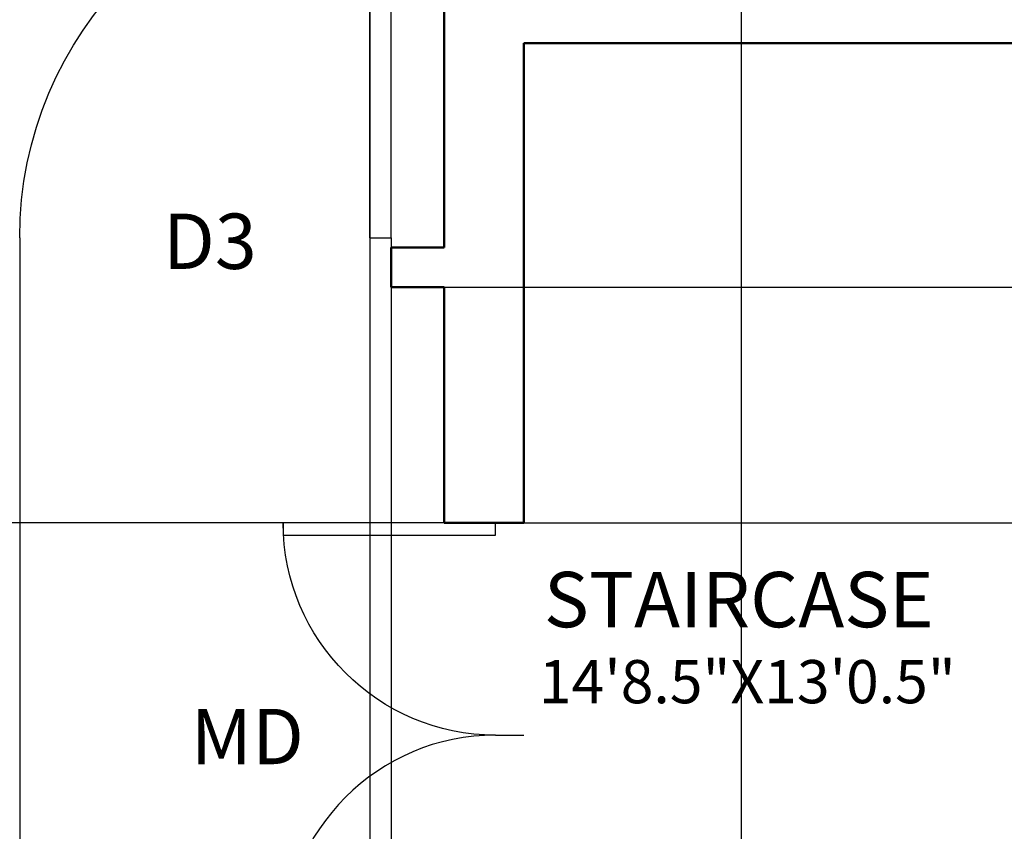
# Model space of a CAD drawing. Units: inches. Extents: x 7359 to 7979, y 33027 to 34263.
# Tile 28 of 32: x 7641 to 7753, y 33841 to 33933. Entities that reach past the tile are written whole.
import ezdxf

# ---------------------------------------------------------------- set-up
doc = ezdxf.new("R2010")
doc.units = ezdxf.units.IN
for name, color, linetype, lineweight in [('A-ANNO-DIMS', 2, 'Continuous', 18), ('A-ANNO-TEXT', 3, 'Continuous', 18), ('A-AREA-IDEN', 7, 'Continuous', 18), ('A-DOOR', 3, 'Continuous', 25), ('A-WALL', 7, 'Continuous', 50)]:
    doc.layers.add(name, color=color, linetype=linetype, lineweight=lineweight)
doc.styles.get("Standard").update_dxf_attribs({"font": 'arial.ttf'})
doc.dimstyles.get("Standard").update_dxf_attribs({"dimtxt": 0.18, "dimasz": 0.18, "dimexe": 0.18, "dimexo": 0.0625, "dimgap": 0.09, "dimtad": 0, "dimtih": 1, "dimtoh": 1, "dimdec": 4, "dimzin": 0, "dimdsep": 46, "dimtxsty": 'Standard', "dimcen": 0.09, "dimadec": 0, "dimazin": 0, "dimtfac": 1, "dimtdec": 4, "dimtofl": 0, "dimtmove": 0, "dimatfit": 3, "dimfxl": 1, "dimtolj": 1, "dimtzin": 0, "dimarcsym": 0})

# ---------------------------------------------------------------- blocks, each defined once
blk = doc.blocks.new('*U2')
for p, q in [((0, 0), (0, -100)), ((750, 0), (750, -100))]:
    blk.add_line(p, q)
blk.add_lwpolyline([(0, 0), (0, 750), (43.75, 750), (43.75, 0)], close=True)
blk.add_arc((0, 0), 750, 0, 90)
blk = doc.blocks.new('*D69')
at = {"layer": 'A-ANNO-DIMS', "color": 0, "lineweight": -2, "transparency": 16777216}
for p, q in [((7681.09, 34081.77), (7681.09, 33632.31)), ((7723.09, 34081.77), (7723.09, 33632.31)), ((7681.27, 33632.49), (7701.87, 33632.49)), ((7722.91, 33632.49), (7702.31, 33632.49))]:
    blk.add_line(p, q, dxfattribs=at)
at = {"layer": 'A-ANNO-DIMS', "color": 0, "transparency": 16777216}
for points in [[(7681.27, 33632.52), (7681.27, 33632.46), (7681.09, 33632.49)], [(7722.91, 33632.52), (7722.91, 33632.46), (7723.09, 33632.49)]]:
    blk.add_solid(points, dxfattribs=at)
at = {"layer": 'Defpoints', "color": 0, "transparency": 16777216}
for p in [(7681.09, 34081.83), (7723.09, 34081.83), (7723.09, 33632.49)]:
    blk.add_point(p, dxfattribs=at)
at = {"layer": 'A-ANNO-DIMS', "color": 0, "transparency": 16777216, "insert": (7702.09, 33632.49), "char_height": 0.18, "attachment_point": 5}
blk.add_mtext('\\A1;42', dxfattribs=at)
blk = doc.blocks.new('*D71')
at = {"layer": 'A-ANNO-DIMS', "color": 0, "lineweight": -2, "transparency": 16777216}
for p, q in [((7641.49, 33907.17), (7641.49, 33632.31)), ((7683.49, 33907.17), (7683.49, 33632.31)), ((7641.67, 33632.49), (7662.27, 33632.49)), ((7683.31, 33632.49), (7662.71, 33632.49))]:
    blk.add_line(p, q, dxfattribs=at)
at = {"layer": 'A-ANNO-DIMS', "color": 0, "transparency": 16777216}
for points in [[(7641.67, 33632.52), (7641.67, 33632.46), (7641.49, 33632.49)], [(7683.31, 33632.52), (7683.31, 33632.46), (7683.49, 33632.49)]]:
    blk.add_solid(points, dxfattribs=at)
at = {"layer": 'Defpoints', "color": 0, "transparency": 16777216}
for p in [(7641.49, 33907.23), (7683.49, 33907.23), (7683.49, 33632.49)]:
    blk.add_point(p, dxfattribs=at)
at = {"layer": 'A-ANNO-DIMS', "color": 0, "transparency": 16777216, "insert": (7662.49, 33632.49), "char_height": 0.18, "attachment_point": 5}
blk.add_mtext('\\A1;42', dxfattribs=at)
blk = doc.blocks.new('*D72')
at = {"layer": 'A-ANNO-DIMS', "color": 0, "lineweight": -2, "transparency": 16777216}
for p, q in [((7689.43, 33876.08), (7359.41, 33876.08)), ((7359.59, 33875.9), (7359.59, 33852.27)), ((7359.59, 33828.26), (7359.59, 33851.9)), ((7689.43, 33828.08), (7359.41, 33828.08))]:
    blk.add_line(p, q, dxfattribs=at)
at = {"layer": 'A-ANNO-DIMS', "color": 0, "transparency": 16777216}
for points in [[(7359.56, 33875.9), (7359.62, 33875.9), (7359.59, 33876.08)], [(7359.56, 33828.26), (7359.62, 33828.26), (7359.59, 33828.08)]]:
    blk.add_solid(points, dxfattribs=at)
at = {"layer": 'Defpoints', "color": 0, "transparency": 16777216}
for p in [(7359.59, 33876.08), (7689.49, 33876.08), (7689.49, 33828.08)]:
    blk.add_point(p, dxfattribs=at)
at = {"layer": 'A-ANNO-DIMS', "color": 0, "transparency": 16777216, "insert": (7359.59, 33852.08), "char_height": 0.18, "attachment_point": 5}
blk.add_mtext('\\A1;48', dxfattribs=at)
blk = doc.blocks.new('*D82')
at = {"layer": 'A-ANNO-DIMS', "color": 0, "lineweight": -2, "transparency": 16777216}
for p, q in [((7689.55, 33902.73), (7968.68, 33902.73)), ((7968.5, 33902.55), (7968.5, 33889.59)), ((7968.5, 33876.26), (7968.5, 33889.23)), ((7689.55, 33876.08), (7968.68, 33876.08))]:
    blk.add_line(p, q, dxfattribs=at)
at = {"layer": 'A-ANNO-DIMS', "color": 0, "transparency": 16777216}
for points in [[(7968.47, 33902.55), (7968.53, 33902.55), (7968.5, 33902.73)], [(7968.47, 33876.26), (7968.53, 33876.26), (7968.5, 33876.08)]]:
    blk.add_solid(points, dxfattribs=at)
at = {"layer": 'Defpoints', "color": 0, "transparency": 16777216}
for p in [(7689.49, 33902.73), (7968.5, 33902.73), (7689.49, 33876.08)]:
    blk.add_point(p, dxfattribs=at)
at = {"layer": 'A-ANNO-DIMS', "color": 0, "transparency": 16777216, "insert": (7968.5, 33889.41), "char_height": 0.18, "attachment_point": 5}
blk.add_mtext('\\A1;26.65', dxfattribs=at)

msp = doc.modelspace()

# ---------------------------------------------------------------- linework, layer by layer
at = {"layer": 'A-WALL'}
for p, q in [((7689.4915, 33939.3339), (7689.4915, 33907.2339)), ((7698.4915, 33930.3339), (7874.9915, 33930.3339)), ((7698.4915, 33930.3339), (7698.4915, 33876.0839)), ((7683.4915, 33907.2339), (7683.4915, 33902.7339)), ((7683.4915, 33907.2339), (7689.4915, 33907.2339)), ((7683.4915, 33902.7339), (7689.4915, 33902.7339)), ((7689.4915, 33902.7339), (7689.4915, 33876.0839)), ((7698.4915, 33876.0839), (7689.4915, 33876.0839))]:
    msp.add_line(p, q, dxfattribs=at)

# ---------------------------------------------------------------- block references
at = {"layer": 'A-DOOR', "xscale": -0.0559999819687567, "yscale": 0.0559999819687567, "zscale": 0.0559999819687567}
msp.add_blockref('*U2', (7683.4915, 33908.3339), dxfattribs=at)
at = {"layer": 'A-DOOR', "yscale": 0.0319999999999999, "zscale": 0.0319999999999999, "rotation": 90}
for p, xscale in [((7695.2915, 33876.0839), -0.0319999999999999), ((7695.2915, 33828.0839), 0.0319999999999999)]:
    msp.add_blockref('*U2', p, dxfattribs=dict(at, xscale=xscale))

# ---------------------------------------------------------------- texts
at = {"layer": 'A-ANNO-TEXT'}
for s, p in [('D3', (7657.6879, 33904.8067)), ('MD', (7660.8244, 33848.7961))]:
    msp.add_text(s, height=6.25941, dxfattribs=at).set_placement(p)
at = {"layer": 'A-AREA-IDEN'}
for s, height, p in [('STAIRCASE', 6.25941, (7700.7699, 33864.2815)), ('14\'8.5"X13\'0.5"', 4.885549, (7700.2067, 33855.6871))]:
    msp.add_text(s, height=height, dxfattribs=at).set_placement(p)

# ---------------------------------------------------------------- dimensions: what is measured, and where the dimension line sits
at = {"layer": 'A-ANNO-DIMS'}
for base, p1, p2, picture, middle in [((7723.0915, 33632.4891), (7681.0915, 34081.8339), (7723.0915, 34081.8339), '*D69', (7702.0915, 33632.4891)), ((7683.4915, 33632.4891), (7641.4915, 33907.2339), (7683.4915, 33907.2339), '*D71', (7662.4915, 33632.4891))]:
    dim = msp.add_linear_dim(base=base, p1=p1, p2=p2, dimstyle='Standard', override={"dimdec": 0, "dimlfac": 1, "dimrnd": 0, "dimzin": 0, "dimdsep": 46, "dimlunit": 2}, dxfattribs=at)
    dim.commit()
    dim.dimension.update_dxf_attribs({"geometry": picture, "text_midpoint": middle})
for base, p1, p2, override, picture, middle in [((7968.502, 33902.7339), (7689.4915, 33876.0839), (7689.4915, 33902.7339), {"dimdec": 2, "dimlfac": 1, "dimrnd": 0, "dimzin": 0, "dimdsep": 46, "dimlunit": 2}, '*D82', (7968.502, 33889.4089)), ((7359.5866, 33876.0839), (7689.4915, 33828.0839), (7689.4915, 33876.0839), {"dimdec": 0, "dimlfac": 1, "dimrnd": 0, "dimzin": 0, "dimdsep": 46, "dimlunit": 2}, '*D72', (7359.5866, 33852.0839))]:
    dim = msp.add_linear_dim(base=base, p1=p1, p2=p2, angle=90, dimstyle='Standard', override=override, dxfattribs=at)
    dim.commit()
    dim.dimension.update_dxf_attribs({"geometry": picture, "text_midpoint": middle})

doc.saveas('drawing.dxf')
